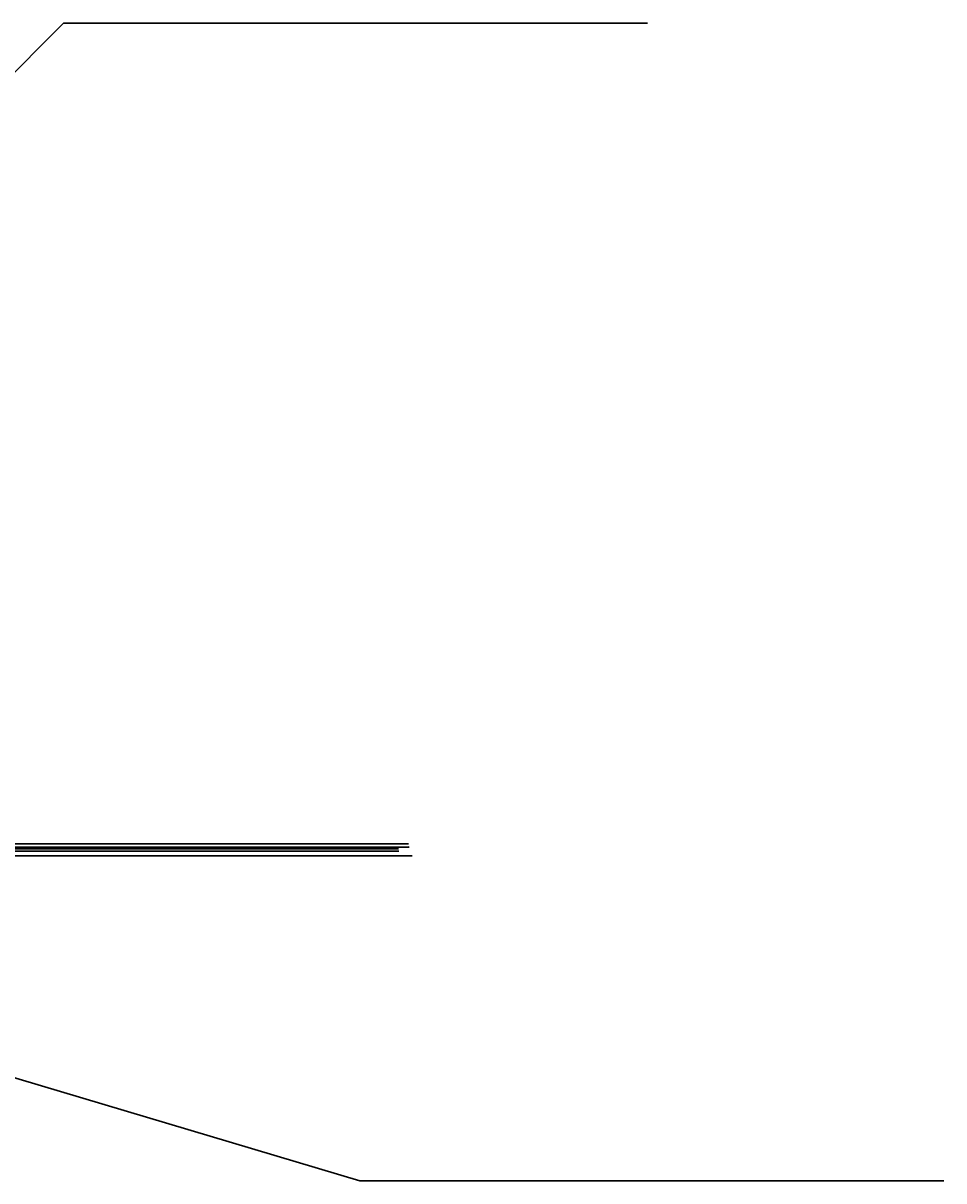
# Model space of a CAD drawing. Units: millimetres. Extents: x -22994 to 29398, y -19990 to 20176.
# Tile 135 of 135: x 13629 to 29398, y -5571 to 14264. Entities that reach past the tile are written whole.
import ezdxf

# ---------------------------------------------------------------- set-up
doc = ezdxf.new("R2010")
doc.units = ezdxf.units.MM
doc.header["$MEASUREMENT"] = 0
doc.layers.add('M-DIMS', color=2, linetype='Continuous', lineweight=18)
doc.styles.get("Standard").update_dxf_attribs({"font": 'arial.ttf'})
doc.dimstyles.get("Standard").update_dxf_attribs({"dimtxt": 0.18, "dimasz": 10000, "dimexe": 0.18, "dimexo": 0.0625, "dimgap": 0.09, "dimtad": 0, "dimtih": 1, "dimtoh": 1, "dimdec": 0, "dimzin": 0, "dimdsep": 46, "dimtxsty": 'Standard', "dimcen": 0.09, "dimadec": 0, "dimazin": 0, "dimtfac": 1, "dimtdec": 0, "dimtofl": 0, "dimtmove": 0, "dimatfit": 3, "dimfxl": 1, "dimtolj": 1, "dimtzin": 0, "dimlwd": 30, "dimarcsym": 0})

# ---------------------------------------------------------------- blocks, each defined once
blk = doc.blocks.new('*D2')
at = {"layer": 'Defpoints', "color": 0, "transparency": 16777216}
for p in [(7, 10), (291, 10), (291, -5)]:
    blk.add_point(p, dxfattribs=at)
at = {"layer": 'M-DIMS', "color": 0, "lineweight": -2, "transparency": 16777216}
for p, q in [((7, 10), (7, -5)), ((291, 10), (291, -5))]:
    blk.add_line(p, q, dxfattribs=at)
at = {"layer": 'M-DIMS', "color": 0, "lineweight": 30, "transparency": 16777216}
for p, q in [((-9993, -5), (-19993, -5)), ((10291, -5), (20291, -5))]:
    blk.add_line(p, q, dxfattribs=at)
at = {"layer": 'M-DIMS', "color": 0, "transparency": 16777216}
for points in [[(-9993, 1662), (-9993, -1672), (7, -5)], [(10291, 1662), (10291, -1672), (291, -5)]]:
    blk.add_solid(points, dxfattribs=at)
at = {"layer": 'M-DIMS', "color": 0, "transparency": 16777216, "insert": (149, -5), "char_height": 0.18, "attachment_point": 5}
blk.add_mtext('\\A1;284.2', dxfattribs=at)
blk = doc.blocks.new('*D3')
at = {"layer": 'Defpoints', "color": 0, "transparency": 16777216}
for p in [(110, 204), (96, 128), (110, 176)]:
    blk.add_point(p, dxfattribs=at)
at = {"layer": 'M-DIMS', "color": 0, "lineweight": 30, "transparency": 16777216}
for p, q in [((-9904, 204), (-19904, 204)), ((10110, 204), (20110, 204))]:
    blk.add_line(p, q, dxfattribs=at)
at = {"layer": 'M-DIMS', "color": 0, "lineweight": -2, "transparency": 16777216}
for p, q in [((96, 128), (96, 204)), ((110, 176), (110, 204))]:
    blk.add_line(p, q, dxfattribs=at)
at = {"layer": 'M-DIMS', "color": 0, "transparency": 16777216}
for points in [[(-9904, 1871), (-9904, -1463), (96, 204)], [(10110, 1871), (10110, -1463), (110, 204)]]:
    blk.add_solid(points, dxfattribs=at)
at = {"layer": 'M-DIMS', "color": 0, "transparency": 16777216, "insert": (103, 204), "char_height": 0.18, "attachment_point": 5}
blk.add_mtext('\\A1;14.432', dxfattribs=at)
blk = doc.blocks.new('*D4')
at = {"layer": 'Defpoints', "color": 0, "transparency": 16777216}
for p in [(116, 204), (110, 176), (116, 176)]:
    blk.add_point(p, dxfattribs=at)
at = {"layer": 'M-DIMS', "color": 0, "lineweight": 30, "transparency": 16777216}
for p, q in [((-9890, 204), (-19890, 204)), ((10116, 204), (20116, 204))]:
    blk.add_line(p, q, dxfattribs=at)
at = {"layer": 'M-DIMS', "color": 0, "lineweight": -2, "transparency": 16777216}
for p, q in [((110, 176), (110, 204)), ((116, 176), (116, 204))]:
    blk.add_line(p, q, dxfattribs=at)
at = {"layer": 'M-DIMS', "color": 0, "transparency": 16777216}
for points in [[(-9890, 1871), (-9890, -1463), (110, 204)], [(10116, 1871), (10116, -1463), (116, 204)]]:
    blk.add_solid(points, dxfattribs=at)
at = {"layer": 'M-DIMS', "color": 0, "transparency": 16777216, "insert": (113, 204), "char_height": 0.18, "attachment_point": 5}
blk.add_mtext('\\A1;6', dxfattribs=at)
blk = doc.blocks.new('*D5')
at = {"layer": 'Defpoints', "color": 0, "transparency": 16777216}
for p in [(181, 204), (116, 176), (181, 176)]:
    blk.add_point(p, dxfattribs=at)
at = {"layer": 'M-DIMS', "color": 0, "lineweight": 30, "transparency": 16777216}
for p, q in [((-9884, 204), (-19884, 204)), ((10181, 204), (20181, 204))]:
    blk.add_line(p, q, dxfattribs=at)
at = {"layer": 'M-DIMS', "color": 0, "lineweight": -2, "transparency": 16777216}
for p, q in [((116, 176), (116, 204)), ((181, 176), (181, 204))]:
    blk.add_line(p, q, dxfattribs=at)
at = {"layer": 'M-DIMS', "color": 0, "transparency": 16777216}
for points in [[(-9884, 1871), (-9884, -1463), (116, 204)], [(10181, 1871), (10181, -1463), (181, 204)]]:
    blk.add_solid(points, dxfattribs=at)
at = {"layer": 'M-DIMS', "color": 0, "transparency": 16777216, "insert": (149, 204), "char_height": 0.18, "attachment_point": 5}
blk.add_mtext('\\A1;65', dxfattribs=at)
blk = doc.blocks.new('*D6')
at = {"layer": 'Defpoints', "color": 0, "transparency": 16777216}
for p in [(187, 204), (181, 176), (187, 176)]:
    blk.add_point(p, dxfattribs=at)
at = {"layer": 'M-DIMS', "color": 0, "lineweight": 30, "transparency": 16777216}
for p, q in [((-9819, 204), (-19819, 204)), ((10187, 204), (20187, 204))]:
    blk.add_line(p, q, dxfattribs=at)
at = {"layer": 'M-DIMS', "color": 0, "lineweight": -2, "transparency": 16777216}
for p, q in [((181, 176), (181, 204)), ((187, 176), (187, 204))]:
    blk.add_line(p, q, dxfattribs=at)
at = {"layer": 'M-DIMS', "color": 0, "transparency": 16777216}
for points in [[(-9819, 1871), (-9819, -1463), (181, 204)], [(10187, 1871), (10187, -1463), (187, 204)]]:
    blk.add_solid(points, dxfattribs=at)
at = {"layer": 'M-DIMS', "color": 0, "transparency": 16777216, "insert": (184, 204), "char_height": 0.18, "attachment_point": 5}
blk.add_mtext('\\A1;6', dxfattribs=at)
blk = doc.blocks.new('*D7')
at = {"layer": 'Defpoints', "color": 0, "transparency": 16777216}
for p in [(202, 204), (187, 176), (202, 128)]:
    blk.add_point(p, dxfattribs=at)
at = {"layer": 'M-DIMS', "color": 0, "lineweight": 30, "transparency": 16777216}
for p, q in [((-9813, 204), (-19813, 204)), ((10202, 204), (20202, 204))]:
    blk.add_line(p, q, dxfattribs=at)
at = {"layer": 'M-DIMS', "color": 0, "lineweight": -2, "transparency": 16777216}
for p, q in [((187, 176), (187, 204)), ((202, 128), (202, 204))]:
    blk.add_line(p, q, dxfattribs=at)
at = {"layer": 'M-DIMS', "color": 0, "transparency": 16777216}
for points in [[(-9813, 1871), (-9813, -1463), (187, 204)], [(10202, 1871), (10202, -1463), (202, 204)]]:
    blk.add_solid(points, dxfattribs=at)
at = {"layer": 'M-DIMS', "color": 0, "transparency": 16777216, "insert": (194, 204), "char_height": 0.18, "attachment_point": 5}
blk.add_mtext('\\A1;14.432', dxfattribs=at)
blk = doc.blocks.new('*D8')
at = {"layer": 'Defpoints', "color": 0, "transparency": 16777216}
for p in [(228, 204), (202, 128), (228, 147)]:
    blk.add_point(p, dxfattribs=at)
at = {"layer": 'M-DIMS', "color": 0, "lineweight": 30, "transparency": 16777216}
for p, q in [((-9798, 204), (-19798, 204)), ((10228, 204), (20228, 204))]:
    blk.add_line(p, q, dxfattribs=at)
at = {"layer": 'M-DIMS', "color": 0, "lineweight": -2, "transparency": 16777216}
for p, q in [((202, 128), (202, 204)), ((228, 147), (228, 204))]:
    blk.add_line(p, q, dxfattribs=at)
at = {"layer": 'M-DIMS', "color": 0, "transparency": 16777216}
for points in [[(-9798, 1871), (-9798, -1463), (202, 204)], [(10228, 1871), (10228, -1463), (228, 204)]]:
    blk.add_solid(points, dxfattribs=at)
at = {"layer": 'M-DIMS', "color": 0, "transparency": 16777216, "insert": (215, 204), "char_height": 0.18, "attachment_point": 5}
blk.add_mtext('\\A1;25.95', dxfattribs=at)
blk = doc.blocks.new('*D10')
at = {"layer": 'Defpoints', "color": 0, "transparency": 16777216}
for p in [(126, 136), (133, 136), (133, -5)]:
    blk.add_point(p, dxfattribs=at)
at = {"layer": 'M-DIMS', "color": 0, "lineweight": -2, "transparency": 16777216}
for p, q in [((126, 136), (126, -5)), ((133, 136), (133, -5))]:
    blk.add_line(p, q, dxfattribs=at)
at = {"layer": 'M-DIMS', "color": 0, "lineweight": 30, "transparency": 16777216}
for p, q in [((-9874, -5), (-19874, -5)), ((10133, -5), (20133, -5))]:
    blk.add_line(p, q, dxfattribs=at)
at = {"layer": 'M-DIMS', "color": 0, "transparency": 16777216}
for points in [[(-9874, 1662), (-9874, -1672), (126, -5)], [(10133, 1662), (10133, -1672), (133, -5)]]:
    blk.add_solid(points, dxfattribs=at)
at = {"layer": 'M-DIMS', "color": 0, "transparency": 16777216, "insert": (129, -5), "char_height": 0.18, "attachment_point": 5}
blk.add_mtext('\\A1;7.696', dxfattribs=at)
blk = doc.blocks.new('*D11')
at = {"layer": 'Defpoints', "color": 0, "transparency": 16777216}
for p in [(133, 136), (136, 136), (136, -5)]:
    blk.add_point(p, dxfattribs=at)
at = {"layer": 'M-DIMS', "color": 0, "lineweight": -2, "transparency": 16777216}
for p, q in [((133, 136), (133, -5)), ((136, 136), (136, -5))]:
    blk.add_line(p, q, dxfattribs=at)
at = {"layer": 'M-DIMS', "color": 0, "lineweight": 30, "transparency": 16777216}
for p, q in [((-9867, -5), (-19867, -5)), ((10136, -5), (20136, -5))]:
    blk.add_line(p, q, dxfattribs=at)
at = {"layer": 'M-DIMS', "color": 0, "transparency": 16777216}
for points in [[(-9867, 1662), (-9867, -1672), (133, -5)], [(10136, 1662), (10136, -1672), (136, -5)]]:
    blk.add_solid(points, dxfattribs=at)
at = {"layer": 'M-DIMS', "color": 0, "transparency": 16777216, "insert": (134, -5), "char_height": 0.18, "attachment_point": 5}
blk.add_mtext('\\A1;2.304', dxfattribs=at)
blk = doc.blocks.new('*D12')
at = {"layer": 'Defpoints', "color": 0, "transparency": 16777216}
for p in [(136, 136), (146, 136), (146, -5)]:
    blk.add_point(p, dxfattribs=at)
at = {"layer": 'M-DIMS', "color": 0, "lineweight": -2, "transparency": 16777216}
for p, q in [((136, 136), (136, -5)), ((146, 136), (146, -5))]:
    blk.add_line(p, q, dxfattribs=at)
at = {"layer": 'M-DIMS', "color": 0, "lineweight": 30, "transparency": 16777216}
for p, q in [((-9864, -5), (-19864, -5)), ((10146, -5), (20146, -5))]:
    blk.add_line(p, q, dxfattribs=at)
at = {"layer": 'M-DIMS', "color": 0, "transparency": 16777216}
for points in [[(-9864, 1662), (-9864, -1672), (136, -5)], [(10146, 1662), (10146, -1672), (146, -5)]]:
    blk.add_solid(points, dxfattribs=at)
at = {"layer": 'M-DIMS', "color": 0, "transparency": 16777216, "insert": (141, -5), "char_height": 0.18, "attachment_point": 5}
blk.add_mtext('\\A1;10', dxfattribs=at)
blk = doc.blocks.new('*D13')
at = {"layer": 'Defpoints', "color": 0, "transparency": 16777216}
for p in [(146, 136), (156, 136), (156, -5)]:
    blk.add_point(p, dxfattribs=at)
at = {"layer": 'M-DIMS', "color": 0, "lineweight": -2, "transparency": 16777216}
for p, q in [((146, 136), (146, -5)), ((156, 136), (156, -5))]:
    blk.add_line(p, q, dxfattribs=at)
at = {"layer": 'M-DIMS', "color": 0, "lineweight": 30, "transparency": 16777216}
for p, q in [((-9854, -5), (-19854, -5)), ((10156, -5), (20156, -5))]:
    blk.add_line(p, q, dxfattribs=at)
at = {"layer": 'M-DIMS', "color": 0, "transparency": 16777216}
for points in [[(-9854, 1662), (-9854, -1672), (146, -5)], [(10156, 1662), (10156, -1672), (156, -5)]]:
    blk.add_solid(points, dxfattribs=at)
at = {"layer": 'M-DIMS', "color": 0, "transparency": 16777216, "insert": (151, -5), "char_height": 0.18, "attachment_point": 5}
blk.add_mtext('\\A1;10', dxfattribs=at)
blk = doc.blocks.new('*D14')
at = {"layer": 'Defpoints', "color": 0, "transparency": 16777216}
for p in [(156, 136), (166, 136), (166, -5)]:
    blk.add_point(p, dxfattribs=at)
at = {"layer": 'M-DIMS', "color": 0, "lineweight": -2, "transparency": 16777216}
for p, q in [((156, 136), (156, -5)), ((166, 136), (166, -5))]:
    blk.add_line(p, q, dxfattribs=at)
at = {"layer": 'M-DIMS', "color": 0, "lineweight": 30, "transparency": 16777216}
for p, q in [((-9844, -5), (-19844, -5)), ((10166, -5), (20166, -5))]:
    blk.add_line(p, q, dxfattribs=at)
at = {"layer": 'M-DIMS', "color": 0, "transparency": 16777216}
for points in [[(-9844, 1662), (-9844, -1672), (156, -5)], [(10166, 1662), (10166, -1672), (166, -5)]]:
    blk.add_solid(points, dxfattribs=at)
at = {"layer": 'M-DIMS', "color": 0, "transparency": 16777216, "insert": (161, -5), "char_height": 0.18, "attachment_point": 5}
blk.add_mtext('\\A1;10', dxfattribs=at)
blk = doc.blocks.new('*D16')
at = {"layer": 'Defpoints', "color": 0, "transparency": 16777216}
for p in [(120, 204), (110, 48), (120, 48)]:
    blk.add_point(p, dxfattribs=at)
at = {"layer": 'M-DIMS', "color": 0, "lineweight": 30, "transparency": 16777216}
for p, q in [((-9890, 204), (-19890, 204)), ((10120, 204), (20120, 204))]:
    blk.add_line(p, q, dxfattribs=at)
at = {"layer": 'M-DIMS', "color": 0, "lineweight": -2, "transparency": 16777216}
for p, q in [((110, 48), (110, 204)), ((120, 48), (120, 204))]:
    blk.add_line(p, q, dxfattribs=at)
at = {"layer": 'M-DIMS', "color": 0, "transparency": 16777216}
for points in [[(-9890, 1871), (-9890, -1463), (110, 204)], [(10120, 1871), (10120, -1463), (120, 204)]]:
    blk.add_solid(points, dxfattribs=at)
at = {"layer": 'M-DIMS', "color": 0, "transparency": 16777216, "insert": (115, 204), "char_height": 0.18, "attachment_point": 5}
blk.add_mtext('\\A1;9.704', dxfattribs=at)
blk = doc.blocks.new('*D17')
at = {"layer": 'Defpoints', "color": 0, "transparency": 16777216}
for p in [(126, 204), (120, 48), (126, 48)]:
    blk.add_point(p, dxfattribs=at)
at = {"layer": 'M-DIMS', "color": 0, "lineweight": 30, "transparency": 16777216}
for p, q in [((-9880, 204), (-19880, 204)), ((10126, 204), (20126, 204))]:
    blk.add_line(p, q, dxfattribs=at)
at = {"layer": 'M-DIMS', "color": 0, "lineweight": -2, "transparency": 16777216}
for p, q in [((120, 48), (120, 204)), ((126, 48), (126, 204))]:
    blk.add_line(p, q, dxfattribs=at)
at = {"layer": 'M-DIMS', "color": 0, "transparency": 16777216}
for points in [[(-9880, 1871), (-9880, -1463), (120, 204)], [(10126, 1871), (10126, -1463), (126, 204)]]:
    blk.add_solid(points, dxfattribs=at)
at = {"layer": 'M-DIMS', "color": 0, "transparency": 16777216, "insert": (123, 204), "char_height": 0.18, "attachment_point": 5}
blk.add_mtext('\\A1;6', dxfattribs=at)
blk = doc.blocks.new('*D18')
at = {"layer": 'Defpoints', "color": 0, "transparency": 16777216}
for p in [(132, 204), (126, 48), (132, 48)]:
    blk.add_point(p, dxfattribs=at)
at = {"layer": 'M-DIMS', "color": 0, "lineweight": 30, "transparency": 16777216}
for p, q in [((-9874, 204), (-19874, 204)), ((10132, 204), (20132, 204))]:
    blk.add_line(p, q, dxfattribs=at)
at = {"layer": 'M-DIMS', "color": 0, "lineweight": -2, "transparency": 16777216}
for p, q in [((126, 48), (126, 204)), ((132, 48), (132, 204))]:
    blk.add_line(p, q, dxfattribs=at)
at = {"layer": 'M-DIMS', "color": 0, "transparency": 16777216}
for points in [[(-9874, 1871), (-9874, -1463), (126, 204)], [(10132, 1871), (10132, -1463), (132, 204)]]:
    blk.add_solid(points, dxfattribs=at)
at = {"layer": 'M-DIMS', "color": 0, "transparency": 16777216, "insert": (129, 204), "char_height": 0.18, "attachment_point": 5}
blk.add_mtext('\\A1;6', dxfattribs=at)
blk = doc.blocks.new('*D19')
at = {"layer": 'Defpoints', "color": 0, "transparency": 16777216}
for p in [(138, 204), (132, 48), (138, 48)]:
    blk.add_point(p, dxfattribs=at)
at = {"layer": 'M-DIMS', "color": 0, "lineweight": 30, "transparency": 16777216}
for p, q in [((-9868, 204), (-19868, 204)), ((10138, 204), (20138, 204))]:
    blk.add_line(p, q, dxfattribs=at)
at = {"layer": 'M-DIMS', "color": 0, "lineweight": -2, "transparency": 16777216}
for p, q in [((132, 48), (132, 204)), ((138, 48), (138, 204))]:
    blk.add_line(p, q, dxfattribs=at)
at = {"layer": 'M-DIMS', "color": 0, "transparency": 16777216}
for points in [[(-9868, 1871), (-9868, -1463), (132, 204)], [(10138, 1871), (10138, -1463), (138, 204)]]:
    blk.add_solid(points, dxfattribs=at)
at = {"layer": 'M-DIMS', "color": 0, "transparency": 16777216, "insert": (135, 204), "char_height": 0.18, "attachment_point": 5}
blk.add_mtext('\\A1;6', dxfattribs=at)
blk = doc.blocks.new('*D20')
at = {"layer": 'Defpoints', "color": 0, "transparency": 16777216}
for p in [(144, 204), (138, 48), (144, 48)]:
    blk.add_point(p, dxfattribs=at)
at = {"layer": 'M-DIMS', "color": 0, "lineweight": 30, "transparency": 16777216}
for p, q in [((-9862, 204), (-19862, 204)), ((10144, 204), (20144, 204))]:
    blk.add_line(p, q, dxfattribs=at)
at = {"layer": 'M-DIMS', "color": 0, "lineweight": -2, "transparency": 16777216}
for p, q in [((138, 48), (138, 204)), ((144, 48), (144, 204))]:
    blk.add_line(p, q, dxfattribs=at)
at = {"layer": 'M-DIMS', "color": 0, "transparency": 16777216}
for points in [[(-9862, 1871), (-9862, -1463), (138, 204)], [(10144, 1871), (10144, -1463), (144, 204)]]:
    blk.add_solid(points, dxfattribs=at)
at = {"layer": 'M-DIMS', "color": 0, "transparency": 16777216, "insert": (141, 204), "char_height": 0.18, "attachment_point": 5}
blk.add_mtext('\\A1;6', dxfattribs=at)
blk = doc.blocks.new('*D21')
at = {"layer": 'Defpoints', "color": 0, "transparency": 16777216}
for p in [(149, 204), (144, 48), (149, 48)]:
    blk.add_point(p, dxfattribs=at)
at = {"layer": 'M-DIMS', "color": 0, "lineweight": 30, "transparency": 16777216}
for p, q in [((-9856, 204), (-19856, 204)), ((10149, 204), (20149, 204))]:
    blk.add_line(p, q, dxfattribs=at)
at = {"layer": 'M-DIMS', "color": 0, "lineweight": -2, "transparency": 16777216}
for p, q in [((144, 48), (144, 204)), ((149, 48), (149, 204))]:
    blk.add_line(p, q, dxfattribs=at)
at = {"layer": 'M-DIMS', "color": 0, "transparency": 16777216}
for points in [[(-9856, 1871), (-9856, -1463), (144, 204)], [(10149, 1871), (10149, -1463), (149, 204)]]:
    blk.add_solid(points, dxfattribs=at)
at = {"layer": 'M-DIMS', "color": 0, "transparency": 16777216, "insert": (147, 204), "char_height": 0.18, "attachment_point": 5}
blk.add_mtext('\\A1;4.945', dxfattribs=at)
blk = doc.blocks.new('*D22')
at = {"layer": 'Defpoints', "color": 0, "transparency": 16777216}
for p in [(149, 31), (155, 31), (155, -5)]:
    blk.add_point(p, dxfattribs=at)
at = {"layer": 'M-DIMS', "color": 0, "lineweight": -2, "transparency": 16777216}
for p, q in [((149, 31), (149, -5)), ((155, 31), (155, -5))]:
    blk.add_line(p, q, dxfattribs=at)
at = {"layer": 'M-DIMS', "color": 0, "lineweight": 30, "transparency": 16777216}
for p, q in [((-9851, -5), (-19851, -5)), ((10155, -5), (20155, -5))]:
    blk.add_line(p, q, dxfattribs=at)
at = {"layer": 'M-DIMS', "color": 0, "transparency": 16777216}
for points in [[(-9851, 1662), (-9851, -1672), (149, -5)], [(10155, 1662), (10155, -1672), (155, -5)]]:
    blk.add_solid(points, dxfattribs=at)
at = {"layer": 'M-DIMS', "color": 0, "transparency": 16777216, "insert": (152, -5), "char_height": 0.18, "attachment_point": 5}
blk.add_mtext('\\A1;6', dxfattribs=at)
blk = doc.blocks.new('*D23')
at = {"layer": 'Defpoints', "color": 0, "transparency": 16777216}
for p in [(155, 31), (161, 31), (161, -5)]:
    blk.add_point(p, dxfattribs=at)
at = {"layer": 'M-DIMS', "color": 0, "lineweight": -2, "transparency": 16777216}
for p, q in [((155, 31), (155, -5)), ((161, 31), (161, -5))]:
    blk.add_line(p, q, dxfattribs=at)
at = {"layer": 'M-DIMS', "color": 0, "lineweight": 30, "transparency": 16777216}
for p, q in [((-9845, -5), (-19845, -5)), ((10161, -5), (20161, -5))]:
    blk.add_line(p, q, dxfattribs=at)
at = {"layer": 'M-DIMS', "color": 0, "transparency": 16777216}
for points in [[(-9845, 1662), (-9845, -1672), (155, -5)], [(10161, 1662), (10161, -1672), (161, -5)]]:
    blk.add_solid(points, dxfattribs=at)
at = {"layer": 'M-DIMS', "color": 0, "transparency": 16777216, "insert": (158, -5), "char_height": 0.18, "attachment_point": 5}
blk.add_mtext('\\A1;6', dxfattribs=at)
blk = doc.blocks.new('*D24')
at = {"layer": 'Defpoints', "color": 0, "transparency": 16777216}
for p in [(161, 31), (166, 31), (166, -5)]:
    blk.add_point(p, dxfattribs=at)
at = {"layer": 'M-DIMS', "color": 0, "lineweight": -2, "transparency": 16777216}
for p, q in [((161, 31), (161, -5)), ((166, 31), (166, -5))]:
    blk.add_line(p, q, dxfattribs=at)
at = {"layer": 'M-DIMS', "color": 0, "lineweight": 30, "transparency": 16777216}
for p, q in [((-9839, -5), (-19839, -5)), ((10166, -5), (20166, -5))]:
    blk.add_line(p, q, dxfattribs=at)
at = {"layer": 'M-DIMS', "color": 0, "transparency": 16777216}
for points in [[(-9839, 1662), (-9839, -1672), (161, -5)], [(10166, 1662), (10166, -1672), (166, -5)]]:
    blk.add_solid(points, dxfattribs=at)
at = {"layer": 'M-DIMS', "color": 0, "transparency": 16777216, "insert": (164, -5), "char_height": 0.18, "attachment_point": 5}
blk.add_mtext('\\A1;5.323', dxfattribs=at)
blk = doc.blocks.new('*D25')
at = {"layer": 'Defpoints', "color": 0, "transparency": 16777216}
for p in [(166, 31), (172, 31), (172, -5)]:
    blk.add_point(p, dxfattribs=at)
at = {"layer": 'M-DIMS', "color": 0, "lineweight": -2, "transparency": 16777216}
for p, q in [((166, 31), (166, -5)), ((172, 31), (172, -5))]:
    blk.add_line(p, q, dxfattribs=at)
at = {"layer": 'M-DIMS', "color": 0, "lineweight": 30, "transparency": 16777216}
for p, q in [((-9834, -5), (-19834, -5)), ((10172, -5), (20172, -5))]:
    blk.add_line(p, q, dxfattribs=at)
at = {"layer": 'M-DIMS', "color": 0, "transparency": 16777216}
for points in [[(-9834, 1662), (-9834, -1672), (166, -5)], [(10172, 1662), (10172, -1672), (172, -5)]]:
    blk.add_solid(points, dxfattribs=at)
at = {"layer": 'M-DIMS', "color": 0, "transparency": 16777216, "insert": (169, -5), "char_height": 0.18, "attachment_point": 5}
blk.add_mtext('\\A1;6', dxfattribs=at)
blk = doc.blocks.new('*D26')
at = {"layer": 'Defpoints', "color": 0, "transparency": 16777216}
for p in [(172, 31), (178, 31), (178, -5)]:
    blk.add_point(p, dxfattribs=at)
at = {"layer": 'M-DIMS', "color": 0, "lineweight": -2, "transparency": 16777216}
for p, q in [((172, 31), (172, -5)), ((178, 31), (178, -5))]:
    blk.add_line(p, q, dxfattribs=at)
at = {"layer": 'M-DIMS', "color": 0, "lineweight": 30, "transparency": 16777216}
for p, q in [((-9828, -5), (-19828, -5)), ((10178, -5), (20178, -5))]:
    blk.add_line(p, q, dxfattribs=at)
at = {"layer": 'M-DIMS', "color": 0, "transparency": 16777216}
for points in [[(-9828, 1662), (-9828, -1672), (172, -5)], [(10178, 1662), (10178, -1672), (178, -5)]]:
    blk.add_solid(points, dxfattribs=at)
at = {"layer": 'M-DIMS', "color": 0, "transparency": 16777216, "insert": (175, -5), "char_height": 0.18, "attachment_point": 5}
blk.add_mtext('\\A1;6', dxfattribs=at)
blk = doc.blocks.new('*D27')
at = {"layer": 'Defpoints', "color": 0, "transparency": 16777216}
for p in [(178, 31), (188, 31), (188, -5)]:
    blk.add_point(p, dxfattribs=at)
at = {"layer": 'M-DIMS', "color": 0, "lineweight": -2, "transparency": 16777216}
for p, q in [((178, 31), (178, -5)), ((188, 31), (188, -5))]:
    blk.add_line(p, q, dxfattribs=at)
at = {"layer": 'M-DIMS', "color": 0, "lineweight": 30, "transparency": 16777216}
for p, q in [((-9822, -5), (-19822, -5)), ((10188, -5), (20188, -5))]:
    blk.add_line(p, q, dxfattribs=at)
at = {"layer": 'M-DIMS', "color": 0, "transparency": 16777216}
for points in [[(-9822, 1662), (-9822, -1672), (178, -5)], [(10188, 1662), (10188, -1672), (188, -5)]]:
    blk.add_solid(points, dxfattribs=at)
at = {"layer": 'M-DIMS', "color": 0, "transparency": 16777216, "insert": (183, -5), "char_height": 0.18, "attachment_point": 5}
blk.add_mtext('\\A1;9.679', dxfattribs=at)
blk = doc.blocks.new('*D29')
at = {"layer": 'Defpoints', "color": 0, "transparency": 16777216}
for p in [(37, 80), (64, 80)]:
    blk.add_point(p, dxfattribs=at)
at = {"layer": 'M-DIMS', "color": 0, "lineweight": -2, "transparency": 16777216}
for q in [(51, 80), (50, 80)]:
    blk.add_line((50, 80), q, dxfattribs=at)
at = {"layer": 'M-DIMS', "color": 0, "lineweight": 30, "transparency": 16777216}
blk.add_line((20064, 80), (10064, 80), dxfattribs=at)
at = {"layer": 'M-DIMS', "color": 0, "transparency": 16777216}
blk.add_solid([(10064, 1747), (10064, -1587), (64, 80)], dxfattribs=at)
at = {"layer": 'M-DIMS', "color": 0, "transparency": 16777216, "insert": (20065, 80), "char_height": 0.18, "attachment_point": 5}
blk.add_mtext('\\A1;∅27.23', dxfattribs=at)
blk = doc.blocks.new('*D30')
at = {"layer": 'Defpoints', "color": 0, "transparency": 16777216}
for p in [(216, 147), (239, 147)]:
    blk.add_point(p, dxfattribs=at)
at = {"layer": 'M-DIMS', "color": 0, "lineweight": -2, "transparency": 16777216}
blk.add_line((228, 147), (228, 147), dxfattribs=at)
blk.add_line((228, 147), (228, 147), dxfattribs=at)
at = {"layer": 'M-DIMS', "color": 0, "lineweight": 30, "transparency": 16777216}
blk.add_line((20239, 147), (10239, 147), dxfattribs=at)
at = {"layer": 'M-DIMS', "color": 0, "transparency": 16777216}
blk.add_solid([(10239, 1814), (10239, -1520), (239, 147)], dxfattribs=at)
at = {"layer": 'M-DIMS', "color": 0, "transparency": 16777216, "insert": (20240, 147), "char_height": 0.18, "attachment_point": 5}
blk.add_mtext('\\A1;∅22.667', dxfattribs=at)
blk = doc.blocks.new('*D31')
at = {"layer": 'Defpoints', "color": 0, "transparency": 16777216}
for p in [(223, 147), (232, 147)]:
    blk.add_point(p, dxfattribs=at)
at = {"layer": 'M-DIMS', "color": 0, "lineweight": -2, "transparency": 16777216}
blk.add_line((228, 147), (228, 147), dxfattribs=at)
blk.add_line((228, 147), (228, 147), dxfattribs=at)
at = {"layer": 'M-DIMS', "color": 0, "lineweight": 30, "transparency": 16777216}
blk.add_line((20232, 149), (10232, 148), dxfattribs=at)
at = {"layer": 'M-DIMS', "color": 0, "transparency": 16777216}
blk.add_solid([(10232, 1814), (10232, -1519), (232, 147)], dxfattribs=at)
at = {"layer": 'M-DIMS', "color": 0, "transparency": 16777216, "insert": (20233, 149), "char_height": 0.18, "attachment_point": 5}
blk.add_mtext('\\A1;∅8.969', dxfattribs=at)
blk = doc.blocks.new('*D33')
at = {"layer": 'Defpoints', "color": 0, "transparency": 16777216}
for p in [(230, 154), (233, 153)]:
    blk.add_point(p, dxfattribs=at)
at = {"layer": 'M-DIMS', "color": 0, "lineweight": -2, "transparency": 16777216}
for p in [(229, 154), (230, 154)]:
    blk.add_line(p, (230, 154), dxfattribs=at)
at = {"layer": 'M-DIMS', "color": 0, "lineweight": 30, "transparency": 16777216}
for p, q in [((19396, -5571), (9815, -2709)), ((29396, -5571), (19396, -5571))]:
    blk.add_line(p, q, dxfattribs=at)
at = {"layer": 'M-DIMS', "color": 0, "transparency": 16777216}
blk.add_solid([(10292, -1112), (9338, -4306), (233, 153)], dxfattribs=at)
at = {"layer": 'M-DIMS', "color": 0, "transparency": 16777216, "insert": (29397, -5571), "char_height": 0.18, "attachment_point": 5}
blk.add_mtext('\\A1;6X R3.586', dxfattribs=at)
blk = doc.blocks.new('*D34')
at = {"layer": 'Defpoints', "color": 0, "transparency": 16777216}
for p in [(177, 121), (179, 123)]:
    blk.add_point(p, dxfattribs=at)
at = {"layer": 'M-DIMS', "color": 0, "lineweight": 30, "transparency": 16777216}
for p, q in [((14322, 14263), (7251, 7193)), ((24322, 14263), (14322, 14263))]:
    blk.add_line(p, q, dxfattribs=at)
at = {"layer": 'M-DIMS', "color": 0, "lineweight": -2, "transparency": 16777216}
blk.add_line((177, 121), (177, 121), dxfattribs=at)
blk.add_line((177, 121), (177, 121), dxfattribs=at)
at = {"layer": 'M-DIMS', "color": 0, "transparency": 16777216}
blk.add_solid([(6072, 8372), (8429, 6014), (179, 123)], dxfattribs=at)
at = {"layer": 'M-DIMS', "color": 0, "transparency": 16777216, "insert": (24323, 14263), "char_height": 0.18, "attachment_point": 5}
blk.add_mtext('\\A1;6X R2.5', dxfattribs=at)
blk = doc.blocks.new('*D37')
at = {"layer": 'Defpoints', "color": 0, "transparency": 16777216}
for p in [(55, 119), (59, 119)]:
    blk.add_point(p, dxfattribs=at)
at = {"layer": 'M-DIMS', "color": 0, "lineweight": -2, "transparency": 16777216}
blk.add_line((57, 119), (57, 119), dxfattribs=at)
blk.add_line((57, 119), (57, 119), dxfattribs=at)
at = {"layer": 'M-DIMS', "color": 0, "lineweight": 30, "transparency": 16777216}
blk.add_line((20059, 116), (10059, 117), dxfattribs=at)
at = {"layer": 'M-DIMS', "color": 0, "transparency": 16777216}
blk.add_solid([(10060, 1784), (10059, -1549), (59, 119)], dxfattribs=at)
at = {"layer": 'M-DIMS', "color": 0, "transparency": 16777216, "insert": (20060, 116), "char_height": 0.18, "attachment_point": 5}
blk.add_mtext('\\A1;∅4.659', dxfattribs=at)

msp = doc.modelspace()

# ---------------------------------------------------------------- dimensions: what is measured, and where the dimension line sits
at = {"layer": 'M-DIMS'}
for center, mpoint, override, picture, middle in [((176.8123, 121.1277), (178.5802, 122.8952), {"dimdec": 1, "dimlfac": 1, "dimrnd": 0, "dimzin": 0, "dimdsep": 46, "dimlunit": 2}, '*D34', (24322.9703, 14263.3108)), ((229.5613, 154.3773), (232.9972, 153.3509), {"dimdec": 3, "dimlfac": 1, "dimrnd": 0, "dimzin": 0, "dimdsep": 46, "dimlunit": 2}, '*D33', (29397.0125, -5570.8378))]:
    dim = msp.add_radius_dim(center=center, mpoint=mpoint, text='6X <>', dimstyle='Standard', override=override, dxfattribs=at)
    dim.commit()
    dim.dimension.update_dxf_attribs({"geometry": picture, "text_midpoint": middle})
for base, p1, p2, override, picture, middle in [((110.2647, 204.1654), (95.8327, 127.967), (110.2647, 176.3662), {"dimdec": 3, "dimlfac": 1, "dimrnd": 0, "dimzin": 0, "dimdsep": 46, "dimlunit": 2}, '*D3', (103.0487, 204.1654)), ((116.2647, 204.1654), (110.2647, 176.3662), (116.2647, 176.3662), {"dimdec": 0, "dimlfac": 1, "dimrnd": 0, "dimzin": 0, "dimdsep": 46, "dimlunit": 2}, '*D4', (113.2647, 204.1654)), ((120.1702, 204.1654), (110.4658, 48.0349), (120.1702, 48.0349), {"dimdec": 3, "dimlfac": 1, "dimrnd": 0, "dimzin": 0, "dimdsep": 46, "dimlunit": 2}, '*D16', (115.318, 204.1654)), ((181.2647, 204.1654), (116.2647, 176.3662), (181.2647, 176.3662), {"dimdec": 0, "dimlfac": 1, "dimrnd": 0, "dimzin": 0, "dimdsep": 46, "dimlunit": 2}, '*D5', (148.7647, 204.1654)), ((126.1702, 204.1654), (120.1702, 48.0349), (126.1702, 48.0349), {"dimdec": 0, "dimlfac": 1, "dimrnd": 0, "dimzin": 0, "dimdsep": 46, "dimlunit": 2}, '*D17', (123.1702, 204.1654)), ((132.1702, 204.1654), (126.1702, 48.0349), (132.1702, 48.0349), {"dimdec": 0, "dimlfac": 1, "dimrnd": 0, "dimzin": 0, "dimdsep": 46, "dimlunit": 2}, '*D18', (129.1702, 204.1654)), ((138.1702, 204.1654), (132.1702, 48.0349), (138.1702, 48.0349), {"dimdec": 0, "dimlfac": 1, "dimrnd": 0, "dimzin": 0, "dimdsep": 46, "dimlunit": 2}, '*D19', (135.1702, 204.1654)), ((144.1702, 204.1654), (138.1702, 48.0349), (144.1702, 48.0349), {"dimdec": 0, "dimlfac": 1, "dimrnd": 0, "dimzin": 0, "dimdsep": 46, "dimlunit": 2}, '*D20', (141.1702, 204.1654)), ((149.11567, 204.16539), (144.17023, 48.03494), (149.11567, 48.03494), {"dimdec": 3, "dimlfac": 1, "dimrnd": 0, "dimzin": 0, "dimdsep": 46, "dimlunit": 2}, '*D21', (146.64295, 204.16539)), ((187.2647, 204.1654), (181.2647, 176.3662), (187.2647, 176.3662), {"dimdec": 0, "dimlfac": 1, "dimrnd": 0, "dimzin": 0, "dimdsep": 46, "dimlunit": 2}, '*D6', (184.2647, 204.1654)), ((201.6967, 204.1654), (187.2647, 176.3662), (201.6967, 127.967), {"dimdec": 3, "dimlfac": 1, "dimrnd": 0, "dimzin": 0, "dimdsep": 46, "dimlunit": 2}, '*D7', (194.4807, 204.1654)), ((227.6485, 204.1654), (201.6967, 127.967), (227.6485, 146.7296), {"dimdec": 2, "dimlfac": 1, "dimrnd": 0, "dimzin": 0, "dimdsep": 46, "dimlunit": 2}, '*D8', (214.6726, 204.1654)), ((290.852, -5.0787), (6.6773, 10.2713), (290.852, 10.2713), {"dimdec": 1, "dimlfac": 1, "dimrnd": 0, "dimzin": 0, "dimdsep": 46, "dimlunit": 2}, '*D2', (148.7647, -5.0787)), ((133.3459, -5.0787), (125.6498, 136.0713), (133.3459, 136.0713), {"dimdec": 3, "dimlfac": 1, "dimrnd": 0, "dimzin": 0, "dimdsep": 46, "dimlunit": 2}, '*D10', (129.4978, -5.0787)), ((135.6498, -5.0787), (133.3459, 136.0713), (135.6498, 136.0713), {"dimdec": 3, "dimlfac": 1, "dimrnd": 0, "dimzin": 0, "dimdsep": 46, "dimlunit": 2}, '*D11', (134.4978, -5.0787)), ((145.6498, -5.0787), (135.6498, 136.0713), (145.6498, 136.0713), {"dimdec": 0, "dimlfac": 1, "dimrnd": 0, "dimzin": 0, "dimdsep": 46, "dimlunit": 2}, '*D12', (140.6498, -5.0787)), ((155.6498, -5.0787), (145.6498, 136.0713), (155.6498, 136.0713), {"dimdec": 0, "dimlfac": 1, "dimrnd": 0, "dimzin": 0, "dimdsep": 46, "dimlunit": 2}, '*D13', (150.6498, -5.0787)), ((155.1157, -5.0787), (149.1157, 30.9895), (155.1157, 30.9895), {"dimdec": 0, "dimlfac": 1, "dimrnd": 0, "dimzin": 0, "dimdsep": 46, "dimlunit": 2}, '*D22', (152.1157, -5.0787)), ((161.1157, -5.0787), (155.1157, 30.9895), (161.1157, 30.9895), {"dimdec": 0, "dimlfac": 1, "dimrnd": 0, "dimzin": 0, "dimdsep": 46, "dimlunit": 2}, '*D23', (158.1157, -5.0787)), ((165.6498, -5.0787), (155.6498, 136.0713), (165.6498, 136.0713), {"dimdec": 0, "dimlfac": 1, "dimrnd": 0, "dimzin": 0, "dimdsep": 46, "dimlunit": 2}, '*D14', (160.6498, -5.0787)), ((166.4387, -5.0787), (161.1157, 30.9895), (166.4387, 30.9895), {"dimdec": 3, "dimlfac": 1, "dimrnd": 0, "dimzin": 0, "dimdsep": 46, "dimlunit": 2}, '*D24', (163.7772, -5.0787)), ((172.4387, -5.0787), (166.4387, 30.9895), (172.4387, 30.9895), {"dimdec": 0, "dimlfac": 1, "dimrnd": 0, "dimzin": 0, "dimdsep": 46, "dimlunit": 2}, '*D25', (169.4387, -5.0787)), ((178.4387, -5.0787), (172.4387, 30.9895), (178.4387, 30.9895), {"dimdec": 0, "dimlfac": 1, "dimrnd": 0, "dimzin": 0, "dimdsep": 46, "dimlunit": 2}, '*D26', (175.4387, -5.0787)), ((188.1175, -5.0787), (178.4387, 30.9895), (188.1175, 30.9895), {"dimdec": 3, "dimlfac": 1, "dimrnd": 0, "dimzin": 0, "dimdsep": 46, "dimlunit": 2}, '*D27', (183.2781, -5.0787))]:
    dim = msp.add_linear_dim(base=base, p1=p1, p2=p2, dimstyle='Standard', override=override, dxfattribs=at)
    dim.commit()
    dim.dimension.update_dxf_attribs({"geometry": picture, "text_midpoint": middle})
for p1, p2, picture, middle in [((216.3148, 146.7291), (238.9821, 146.73), '*D30', (20238.9821, 147.4959)), ((223.1641, 146.7291), (232.1328, 146.73), '*D31', (20232.1327, 148.6656))]:
    dim = msp.add_diameter_dim_2p(p1=p1, p2=p2, dimstyle='Standard', override={"dimdec": 3, "dimlfac": 1, "dimrnd": 0, "dimzin": 0, "dimdsep": 46, "dimlunit": 2}, dxfattribs=at)
    dim.commit()
    dim.dimension.update_dxf_attribs({"geometry": picture, "text_midpoint": middle, "dimtype": 163})
for p1, p2, override, picture, middle in [((36.8006, 80.045), (64.0296, 80.045), {"dimdec": 2, "dimlfac": 1, "dimrnd": 0, "dimzin": 0, "dimdsep": 46, "dimlunit": 2}, '*D29', (20064.0296, 80.0303)), ((54.8343, 118.6145), (59.4936, 118.614), {"dimdec": 3, "dimlfac": 1, "dimrnd": 0, "dimzin": 0, "dimdsep": 46, "dimlunit": 2}, '*D37', (20059.4934, 116.2531))]:
    dim = msp.add_diameter_dim_2p(p1=p1, p2=p2, dimstyle='Standard', override=override, dxfattribs=at)
    dim.commit()
    dim.dimension.update_dxf_attribs({"geometry": picture, "text_midpoint": middle})

doc.saveas('drawing.dxf')
